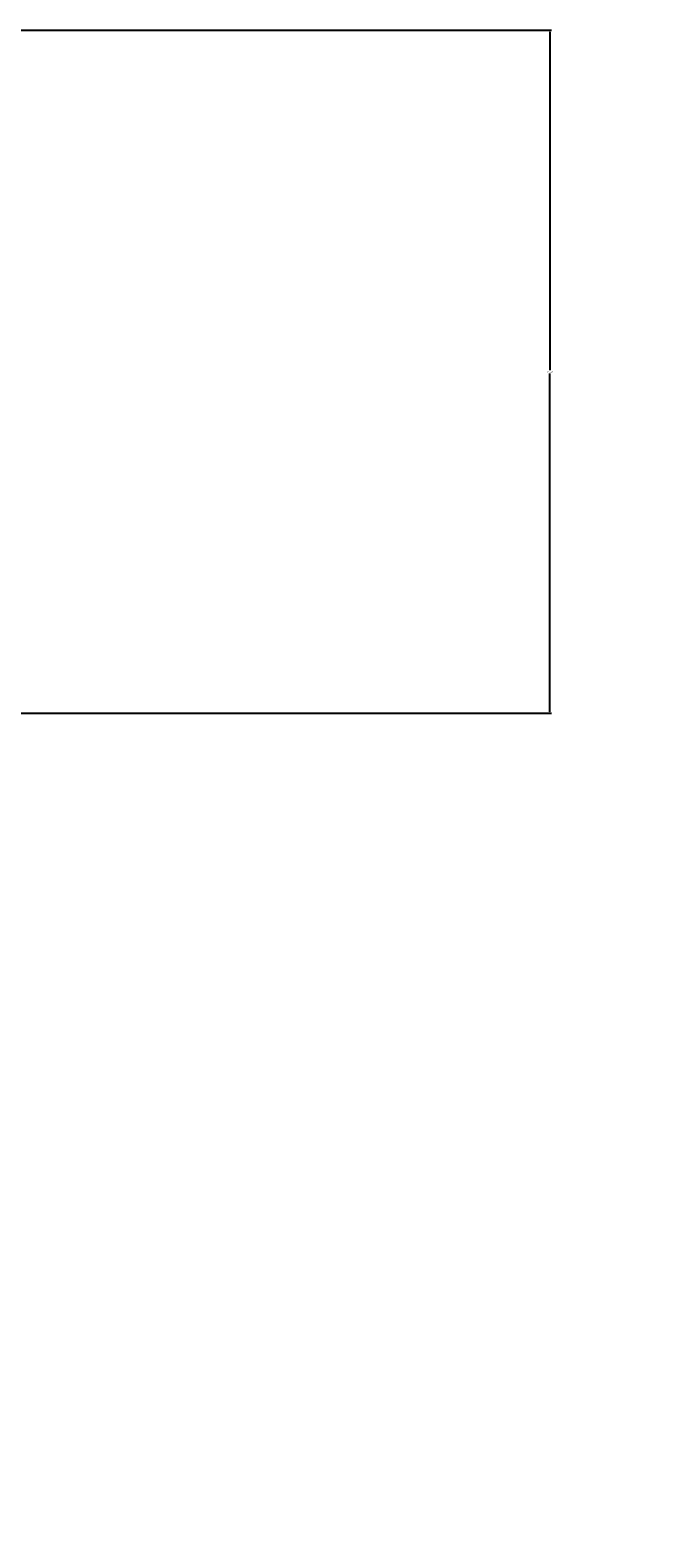
# Model space of a CAD drawing. Units: inches. Extents: x -46 to 1145, y -527 to 760.
# Tile 7 of 57: x 504 to 573, y -435 to -270. Entities that reach past the tile are written whole.
import ezdxf

# ---------------------------------------------------------------- set-up
doc = ezdxf.new("R2010")
doc.units = ezdxf.units.IN
doc.header["$MEASUREMENT"] = 0
doc.layers.add('A-ANNO-DIMS', color=2, linetype='Continuous', lineweight=18)
doc.styles.get("Standard").update_dxf_attribs({"font": 'arial.ttf'})
doc.dimstyles.get("Standard").update_dxf_attribs({"dimtxt": 0.18, "dimasz": 0.18, "dimexe": 0.18, "dimexo": 0.0625, "dimgap": 0.09, "dimtad": 0, "dimtih": 1, "dimtoh": 1, "dimdec": 0, "dimzin": 0, "dimdsep": 46, "dimlunit": 3, "dimtxsty": 'Standard', "dimcen": 0.09, "dimadec": 0, "dimazin": 0, "dimtfac": 1, "dimtdec": 0, "dimtofl": 0, "dimtmove": 0, "dimatfit": 3, "dimfxl": 1, "dimtolj": 1, "dimtzin": 0, "dimarcsym": 0})

# ---------------------------------------------------------------- blocks, each defined once
blk = doc.blocks.new('*D700')
at = {"layer": 'A-ANNO-DIMS', "color": 0, "lineweight": -2, "transparency": 16777216}
for p, q in [((501.79, -270.48), (560.51, -270.48)), ((560.33, -270.66), (560.33, -307.56)), ((560.33, -344.82), (560.33, -307.92)), ((501.79, -345), (560.51, -345))]:
    blk.add_line(p, q, dxfattribs=at)
at = {"layer": 'A-ANNO-DIMS', "color": 0, "transparency": 16777216}
for points in [[(560.3, -270.66), (560.36, -270.66), (560.33, -270.48)], [(560.3, -344.82), (560.36, -344.82), (560.33, -345)]]:
    blk.add_solid(points, dxfattribs=at)
at = {"layer": 'Defpoints', "color": 0, "transparency": 16777216}
for p in [(501.73, -270.48), (501.73, -345), (560.33, -345)]:
    blk.add_point(p, dxfattribs=at)
at = {"layer": 'A-ANNO-DIMS', "color": 0, "transparency": 16777216, "insert": (560.33, -307.74), "char_height": 0.18, "attachment_point": 5}
blk.add_mtext('\\A1;74.52', dxfattribs=at)
blk = doc.blocks.new('*D702')
at = {"layer": 'A-ANNO-DIMS', "color": 0, "lineweight": -2, "transparency": 16777216}
for p, q in [((189.63, -39.48), (1145.34, -39.48)), ((1145.16, -39.66), (1145.16, -249.3)), ((1145.16, -459.3), (1145.16, -249.66)), ((183.63, -459.48), (1145.34, -459.48))]:
    blk.add_line(p, q, dxfattribs=at)
at = {"layer": 'A-ANNO-DIMS', "color": 0, "transparency": 16777216}
for points in [[(1145.13, -39.66), (1145.19, -39.66), (1145.16, -39.48)], [(1145.13, -459.3), (1145.19, -459.3), (1145.16, -459.48)]]:
    blk.add_solid(points, dxfattribs=at)
at = {"layer": 'Defpoints', "color": 0, "transparency": 16777216}
for p in [(189.56, -39.48), (1145.16, -39.48), (183.56, -459.48)]:
    blk.add_point(p, dxfattribs=at)
at = {"layer": 'A-ANNO-DIMS', "color": 0, "transparency": 16777216, "insert": (1145.16, -249.48), "char_height": 0.18, "attachment_point": 5}
blk.add_mtext('\\A1;420', dxfattribs=at)

msp = doc.modelspace()

# ---------------------------------------------------------------- dimensions: what is measured, and where the dimension line sits
at = {"layer": 'A-ANNO-DIMS'}
for base, p1, p2, angle, override, picture, middle in [((1145.1637, -39.4824), (183.5637, -459.4824), (189.5637, -39.4824), 90, {"dimdec": 0, "dimlfac": 1, "dimrnd": 0, "dimzin": 0, "dimdsep": 46, "dimlunit": 2}, '*D702', (1145.1637, -249.4824)), ((560.3297, -345.0009), (501.7297, -270.4792), (501.7297, -345.0009), 270, {"dimdec": 2, "dimlfac": 1, "dimrnd": 0, "dimzin": 0, "dimdsep": 46, "dimlunit": 2}, '*D700', (560.3297, -307.74))]:
    dim = msp.add_linear_dim(base=base, p1=p1, p2=p2, angle=angle, dimstyle='Standard', override=override, dxfattribs=at)
    dim.commit()
    dim.dimension.update_dxf_attribs({"geometry": picture, "text_midpoint": middle})

doc.saveas('drawing.dxf')
